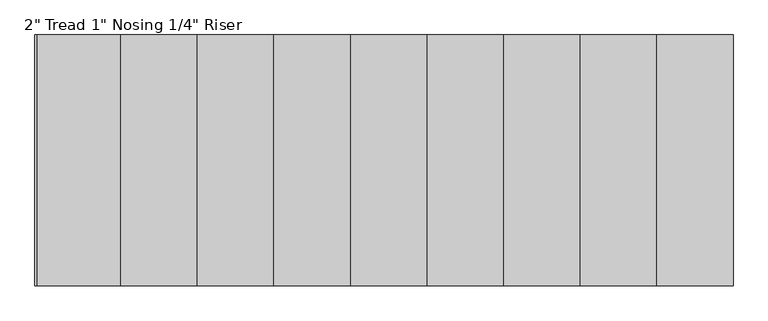
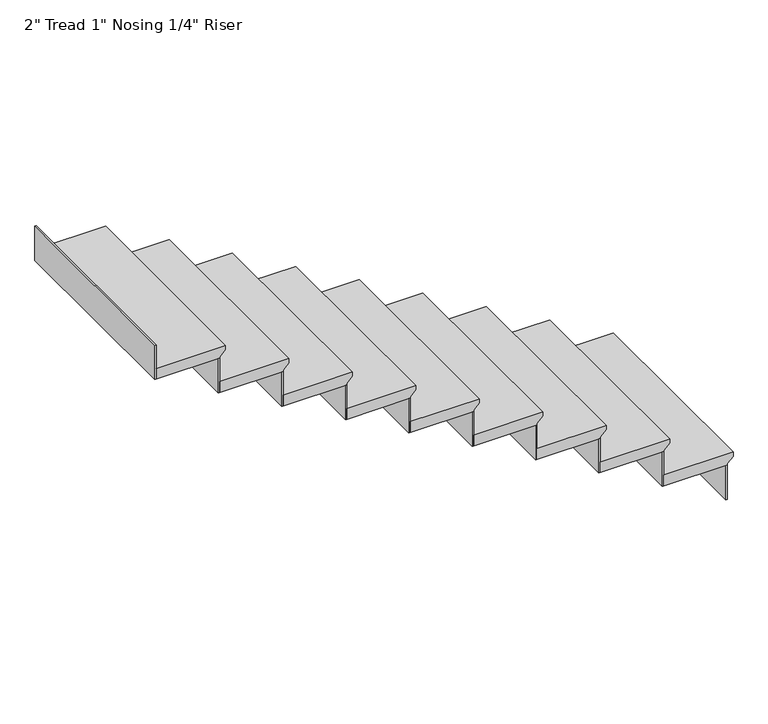
"""IFC4 building model written with IfcOpenShell, lengths in millimetres: stair flight geometry."""

from ifc_helpers import new_model, si_unit, frame, origin, place, context, project, spatial, polyline, outline, extrude, source, transform, mapped, element, save


def stair_flight_e10c2242(model_context):
    return source(origin(), model_context, "Body", "SweptSolid", [
        extrude(outline(polyline([(11361.42, 923.4845537), (11361.42, 618.6845537), (11310.62, 618.6845537), (11310.62, 898.0845537), (11316.97, 898.0845537), (11342.37, 923.4845537), (11361.42, 923.4845537)])), frame((0.0, -5753.3544725, 0.0), z_axis=(0.0, 1.0, 0.0), x_axis=(0.0, 0.0, 1.0)), (0.0, 0.0, 1.0), 914.4),
        extrude(outline(polyline([(891.7345537, -4838.9544725), (898.0845537, -4838.9544725), (898.0845537, -5753.3544725), (891.7345537, -5753.3544725), (891.7345537, -4838.9544725)])), frame((0.0, 0.0, 11150.6), z_axis=(0.0, 0.0, 1.0), x_axis=(1.0, 0.0, 0.0)), (0.0, 0.0, 1.0), 160.02),
        extrude(outline(polyline([(612.3345537, -4838.9544725), (618.6845537, -4838.9544725), (618.6845537, -5753.3544725), (612.3345537, -5753.3544725), (612.3345537, -4838.9544725)])), frame((0.0, 0.0, 11310.62), z_axis=(0.0, 0.0, 1.0), x_axis=(1.0, 0.0, 0.0)), (0.0, 0.0, 1.0), 160.02),
        extrude(outline(polyline([(11521.44, 644.0845537), (11521.44, 339.2845537), (11470.64, 339.2845537), (11470.64, 618.6845537), (11476.99, 618.6845537), (11502.39, 644.0845537), (11521.44, 644.0845537)])), frame((0.0, -5753.3544725, 0.0), z_axis=(0.0, 1.0, 0.0), x_axis=(0.0, 0.0, 1.0)), (0.0, 0.0, 1.0), 914.4),
        extrude(outline(polyline([(332.9345537, -4838.9544725), (339.2845537, -4838.9544725), (339.2845537, -5753.3544725), (332.9345537, -5753.3544725), (332.9345537, -4838.9544725)])), frame((0.0, 0.0, 11470.64), z_axis=(0.0, 0.0, 1.0), x_axis=(1.0, 0.0, 0.0)), (0.0, 0.0, 1.0), 160.02),
        extrude(outline(polyline([(11681.46, 364.6845537), (11681.46, 59.8845537), (11630.66, 59.8845537), (11630.66, 339.2845537), (11637.01, 339.2845537), (11662.41, 364.6845537), (11681.46, 364.6845537)])), frame((0.0, -5753.3544725, 0.0), z_axis=(0.0, 1.0, 0.0), x_axis=(0.0, 0.0, 1.0)), (0.0, 0.0, 1.0), 914.4),
        extrude(outline(polyline([(53.5345537, -4838.9544725), (59.8845537, -4838.9544725), (59.8845537, -5753.3544725), (53.5345537, -5753.3544725), (53.5345537, -4838.9544725)])), frame((0.0, 0.0, 11630.66), z_axis=(0.0, 0.0, 1.0), x_axis=(1.0, 0.0, 0.0)), (0.0, 0.0, 1.0), 160.02),
        extrude(outline(polyline([(11841.48, 85.2845537), (11841.48, -219.5154463), (11790.68, -219.5154463), (11790.68, 59.8845537), (11797.03, 59.8845537), (11822.43, 85.2845537), (11841.48, 85.2845537)])), frame((0.0, -5753.3544725, 0.0), z_axis=(0.0, 1.0, 0.0), x_axis=(0.0, 0.0, 1.0)), (0.0, 0.0, 1.0), 914.4),
        extrude(outline(polyline([(-225.8654463, -4838.9544725), (-219.5154463, -4838.9544725), (-219.5154463, -5753.3544725), (-225.8654463, -5753.3544725), (-225.8654463, -4838.9544725)])), frame((0.0, 0.0, 11790.68), z_axis=(0.0, 0.0, 1.0), x_axis=(1.0, 0.0, 0.0)), (0.0, 0.0, 1.0), 160.02),
        extrude(outline(polyline([(12001.5, -194.1154463), (12001.5, -498.9154463), (11950.7, -498.9154463), (11950.7, -219.5154463), (11957.05, -219.5154463), (11982.45, -194.1154463), (12001.5, -194.1154463)])), frame((0.0, -5753.3544725, 0.0), z_axis=(0.0, 1.0, 0.0), x_axis=(0.0, 0.0, 1.0)), (0.0, 0.0, 1.0), 914.4),
        extrude(outline(polyline([(-505.2654463, -4838.9544725), (-498.9154463, -4838.9544725), (-498.9154463, -5753.3544725), (-505.2654463, -5753.3544725), (-505.2654463, -4838.9544725)])), frame((0.0, 0.0, 11950.7), z_axis=(0.0, 0.0, 1.0), x_axis=(1.0, 0.0, 0.0)), (0.0, 0.0, 1.0), 160.02),
        extrude(outline(polyline([(12161.52, -473.5154463), (12161.52, -778.3154463), (12110.72, -778.3154463), (12110.72, -498.9154463), (12117.07, -498.9154463), (12142.47, -473.5154463), (12161.52, -473.5154463)])), frame((0.0, -5753.3544725, 0.0), z_axis=(0.0, 1.0, 0.0), x_axis=(0.0, 0.0, 1.0)), (0.0, 0.0, 1.0), 914.4),
        extrude(outline(polyline([(-784.6654463, -4838.9544725), (-778.3154463, -4838.9544725), (-778.3154463, -5753.3544725), (-784.6654463, -5753.3544725), (-784.6654463, -4838.9544725)])), frame((0.0, 0.0, 12110.72), z_axis=(0.0, 0.0, 1.0), x_axis=(1.0, 0.0, 0.0)), (0.0, 0.0, 1.0), 160.02),
        extrude(outline(polyline([(12321.54, -752.9154463), (12321.54, -1057.7154463), (12270.74, -1057.7154463), (12270.74, -778.3154463), (12277.09, -778.3154463), (12302.49, -752.9154463), (12321.54, -752.9154463)])), frame((0.0, -5753.3544725, 0.0), z_axis=(0.0, 1.0, 0.0), x_axis=(0.0, 0.0, 1.0)), (0.0, 0.0, 1.0), 914.4),
        extrude(outline(polyline([(-1064.0654463, -4838.9544725), (-1057.7154463, -4838.9544725), (-1057.7154463, -5753.3544725), (-1064.0654463, -5753.3544725), (-1064.0654463, -4838.9544725)])), frame((0.0, 0.0, 12270.74), z_axis=(0.0, 0.0, 1.0), x_axis=(1.0, 0.0, 0.0)), (0.0, 0.0, 1.0), 160.02),
        extrude(outline(polyline([(12481.56, -1032.3154463), (12481.56, -1337.1154463), (12430.76, -1337.1154463), (12430.76, -1057.7154463), (12437.11, -1057.7154463), (12462.51, -1032.3154463), (12481.56, -1032.3154463)])), frame((0.0, -5753.3544725, 0.0), z_axis=(0.0, 1.0, 0.0), x_axis=(0.0, 0.0, 1.0)), (0.0, 0.0, 1.0), 914.4),
        extrude(outline(polyline([(-1343.4654463, -4838.9544725), (-1337.1154463, -4838.9544725), (-1337.1154463, -5753.3544725), (-1343.4654463, -5753.3544725), (-1343.4654463, -4838.9544725)])), frame((0.0, 0.0, 12430.76), z_axis=(0.0, 0.0, 1.0), x_axis=(1.0, 0.0, 0.0)), (0.0, 0.0, 1.0), 160.02),
        extrude(outline(polyline([(-1622.8654463, -4838.9544725), (-1616.5154463, -4838.9544725), (-1616.5154463, -5753.3544725), (-1622.8654463, -5753.3544725), (-1622.8654463, -4838.9544725)])), frame((0.0, 0.0, 12590.78), z_axis=(0.0, 0.0, 1.0), x_axis=(1.0, 0.0, 0.0)), (0.0, 0.0, 1.0), 160.02),
        extrude(outline(polyline([(12641.58, -1311.7154463), (12641.58, -1616.5154463), (12590.78, -1616.5154463), (12590.78, -1337.1154463), (12597.13, -1337.1154463), (12622.53, -1311.7154463), (12641.58, -1311.7154463)])), frame((0.0, -5753.3544725, 0.0), z_axis=(0.0, 1.0, 0.0), x_axis=(0.0, 0.0, 1.0)), (0.0, 0.0, 1.0), 914.4),
    ])


if __name__ == "__main__":
    model = new_model("IFC4")
    model_context = context("Model", 3, world=origin())
    ifc_project = project(units=[si_unit("LENGTHUNIT", "METRE", prefix="MILLI")], contexts=[model_context])
    site = spatial("IfcSite", under=ifc_project)
    building = spatial("IfcBuilding", under=site)
    placement = place(None, origin())
    stair_flight_shape = stair_flight_e10c2242(model_context)
    element("IfcStairFlight", 1, ObjectType="2\" Tread 1\" Nosing 1/4\" Riser", at=placement, inside=building, context=model_context, shape_type="MappedRepresentation", body=[
        mapped(stair_flight_shape, transform((0.0, 0.0, 0.0), x_axis=(1.0, 0.0, 0.0), y_axis=(0.0, 1.0, 0.0), z_axis=(0.0, 0.0, 1.0))),
    ])
    save(model, "model.ifc")
